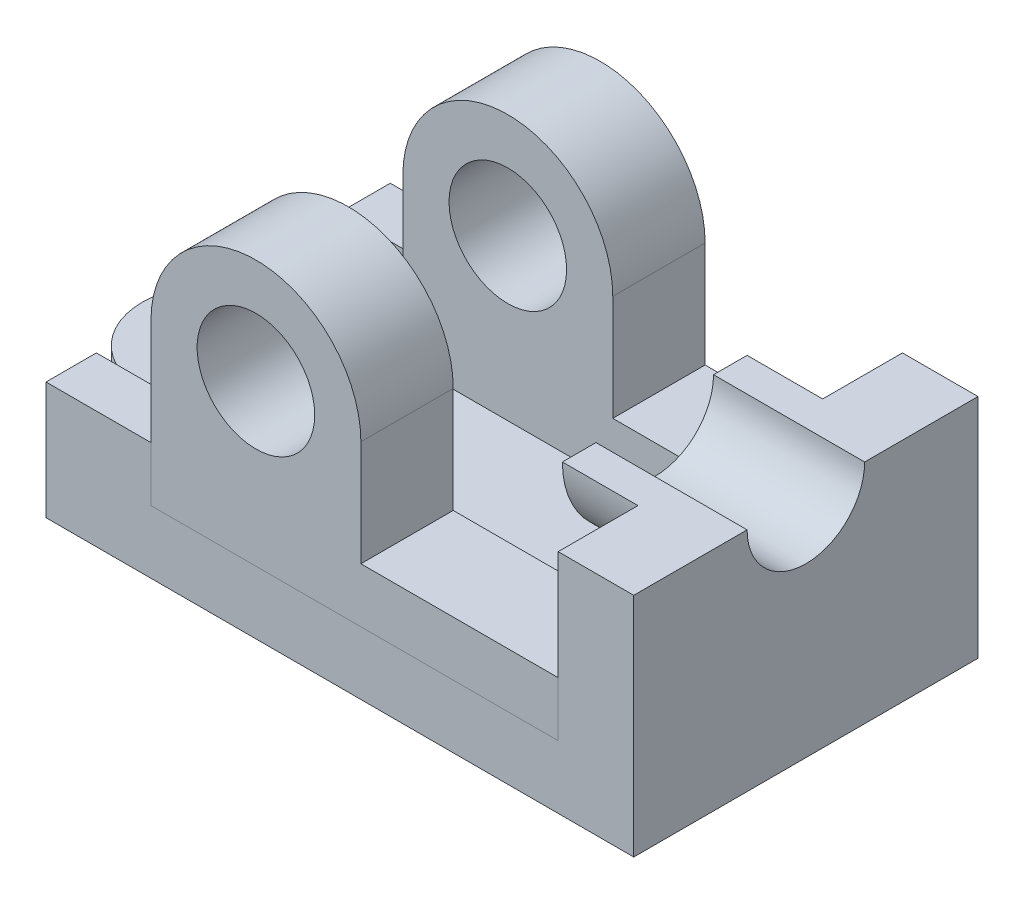
ISO-10303-21;
HEADER;
FILE_DESCRIPTION(('STEP AP214'),'2;1');
FILE_NAME('part.step','',(''),(''),'','','');
FILE_SCHEMA(('AUTOMOTIVE_DESIGN { 1 0 10303 214 1 1 1 1 }'));
ENDSEC;
DATA;
#1=APPLICATION_CONTEXT('core data for automotive mechanical design processes');
#2=APPLICATION_PROTOCOL_DEFINITION('international standard','automotive_design',2000,#1);
#3=PRODUCT_CONTEXT('',#1,'mechanical');
#4=PRODUCT('Part','Part','',(#3));
#5=PRODUCT_RELATED_PRODUCT_CATEGORY('part','',(#4));
#6=PRODUCT_DEFINITION_FORMATION('','',#4);
#7=PRODUCT_DEFINITION_CONTEXT('part definition',#1,'design');
#8=PRODUCT_DEFINITION('design','',#6,#7);
#9=PRODUCT_DEFINITION_SHAPE('','',#8);
#10=(LENGTH_UNIT() NAMED_UNIT(*) SI_UNIT(.MILLI.,.METRE.));
#11=(NAMED_UNIT(*) PLANE_ANGLE_UNIT() SI_UNIT($,.RADIAN.));
#12=(NAMED_UNIT(*) SI_UNIT($,.STERADIAN.) SOLID_ANGLE_UNIT());
#13=UNCERTAINTY_MEASURE_WITH_UNIT(LENGTH_MEASURE(1.E-05),#10,'distance_accuracy_value','');
#14=(GEOMETRIC_REPRESENTATION_CONTEXT(3) GLOBAL_UNCERTAINTY_ASSIGNED_CONTEXT((#13)) GLOBAL_UNIT_ASSIGNED_CONTEXT((#10,
#11,#12)) REPRESENTATION_CONTEXT('',''));
#15=CARTESIAN_POINT('',(0.,0.,0.));
#16=DIRECTION('',(0.,0.,1.));
#17=DIRECTION('',(1.,0.,0.));
#18=AXIS2_PLACEMENT_3D('',#15,#16,#17);
#19=CARTESIAN_POINT('',(-20.,45.6684675281199,19.));
#20=DIRECTION('',(0.,0.,1.));
#21=DIRECTION('',(1.,0.,0.));
#22=AXIS2_PLACEMENT_3D('',#19,#20,#21);
#23=CYLINDRICAL_SURFACE('',#22,25.);
#24=CARTESIAN_POINT('',(-20.,45.6684675281199,41.));
#25=DIRECTION('',(0.,0.,1.));
#26=DIRECTION('',(1.,0.,0.));
#27=AXIS2_PLACEMENT_3D('',#24,#25,#26);
#28=CIRCLE('',#27,25.);
#29=CARTESIAN_POINT('',(5.,45.6684675281199,41.));
#30=VERTEX_POINT('',#29);
#31=CARTESIAN_POINT('',(-45.,45.6684675281199,41.));
#32=VERTEX_POINT('',#31);
#33=EDGE_CURVE('E137',#30,#32,#28,.T.);
#34=ORIENTED_EDGE('',*,*,#33,.F.);
#35=DIRECTION('',(0.,0.,1.));
#36=VECTOR('',#35,1.);
#37=CARTESIAN_POINT('',(5.,45.6684675281199,19.));
#38=LINE('',#37,#36);
#39=CARTESIAN_POINT('',(5.,45.6684675281199,19.));
#40=VERTEX_POINT('',#39);
#41=EDGE_CURVE('E12',#40,#30,#38,.T.);
#42=ORIENTED_EDGE('',*,*,#41,.F.);
#43=CARTESIAN_POINT('',(-20.,45.6684675281199,19.));
#44=DIRECTION('',(0.,0.,1.));
#45=DIRECTION('',(1.,0.,0.));
#46=AXIS2_PLACEMENT_3D('',#43,#44,#45);
#47=CIRCLE('',#46,25.);
#48=CARTESIAN_POINT('',(-45.,45.6684675281199,19.));
#49=VERTEX_POINT('',#48);
#50=EDGE_CURVE('E155',#40,#49,#47,.T.);
#51=ORIENTED_EDGE('',*,*,#50,.T.);
#52=DIRECTION('',(0.,0.,1.));
#53=VECTOR('',#52,1.);
#54=CARTESIAN_POINT('',(-45.,45.6684675281199,19.));
#55=LINE('',#54,#53);
#56=EDGE_CURVE('E103',#49,#32,#55,.T.);
#57=ORIENTED_EDGE('',*,*,#56,.T.);
#58=EDGE_LOOP('',(#34,#42,#51,#57));
#59=FACE_BOUND('',#58,.T.);
#60=ADVANCED_FACE('F51',(#59),#23,.T.);
#61=CARTESIAN_POINT('',(5.,45.6684675281199,19.));
#62=DIRECTION('',(1.,0.,0.));
#63=DIRECTION('',(0.,1.,0.));
#64=AXIS2_PLACEMENT_3D('',#61,#62,#63);
#65=PLANE('',#64);
#66=DIRECTION('',(0.,1.,0.));
#67=VECTOR('',#66,1.);
#68=CARTESIAN_POINT('',(5.,45.6684675281199,41.));
#69=LINE('',#68,#67);
#70=CARTESIAN_POINT('',(5.,20.5,41.));
#71=VERTEX_POINT('',#70);
#72=EDGE_CURVE('E148',#71,#30,#69,.T.);
#73=ORIENTED_EDGE('',*,*,#72,.F.);
#74=DIRECTION('',(0.,0.,1.));
#75=VECTOR('',#74,1.);
#76=CARTESIAN_POINT('',(5.,20.5,19.));
#77=LINE('',#76,#75);
#78=CARTESIAN_POINT('',(5.,20.5,19.));
#79=VERTEX_POINT('',#78);
#80=EDGE_CURVE('E58',#79,#71,#77,.T.);
#81=ORIENTED_EDGE('',*,*,#80,.F.);
#82=DIRECTION('',(0.,1.,0.));
#83=VECTOR('',#82,1.);
#84=CARTESIAN_POINT('',(5.,45.6684675281199,19.));
#85=LINE('',#84,#83);
#86=EDGE_CURVE('E130',#79,#40,#85,.T.);
#87=ORIENTED_EDGE('',*,*,#86,.T.);
#88=ORIENTED_EDGE('',*,*,#41,.T.);
#89=EDGE_LOOP('',(#73,#81,#87,#88));
#90=FACE_BOUND('',#89,.T.);
#91=ADVANCED_FACE('F163',(#90),#65,.T.);
#92=CARTESIAN_POINT('',(5.,20.5,19.));
#93=DIRECTION('',(0.,1.,0.));
#94=DIRECTION('',(0.,0.,1.));
#95=AXIS2_PLACEMENT_3D('',#92,#93,#94);
#96=PLANE('',#95);
#97=DIRECTION('',(-1.,0.,0.));
#98=VECTOR('',#97,1.);
#99=CARTESIAN_POINT('',(5.,20.5,41.));
#100=LINE('',#99,#98);
#101=CARTESIAN_POINT('',(52.,20.5,41.));
#102=VERTEX_POINT('',#101);
#103=EDGE_CURVE('E112',#102,#71,#100,.T.);
#104=ORIENTED_EDGE('',*,*,#103,.F.);
#105=DIRECTION('',(0.,0.,1.));
#106=VECTOR('',#105,1.);
#107=CARTESIAN_POINT('',(52.,20.5,19.));
#108=LINE('',#107,#106);
#109=CARTESIAN_POINT('',(52.,20.5,19.));
#110=VERTEX_POINT('',#109);
#111=EDGE_CURVE('E107',#110,#102,#108,.T.);
#112=ORIENTED_EDGE('',*,*,#111,.F.);
#113=DIRECTION('',(-1.,0.,0.));
#114=VECTOR('',#113,1.);
#115=CARTESIAN_POINT('',(5.,20.5,19.));
#116=LINE('',#115,#114);
#117=EDGE_CURVE('E115',#110,#79,#116,.T.);
#118=ORIENTED_EDGE('',*,*,#117,.T.);
#119=ORIENTED_EDGE('',*,*,#80,.T.);
#120=EDGE_LOOP('',(#104,#112,#118,#119));
#121=FACE_BOUND('',#120,.T.);
#122=ADVANCED_FACE('F111',(#121),#96,.T.);
#123=CARTESIAN_POINT('',(52.,20.5,19.));
#124=DIRECTION('',(1.,0.,0.));
#125=DIRECTION('',(0.,0.,-1.));
#126=AXIS2_PLACEMENT_3D('',#123,#124,#125);
#127=PLANE('',#126);
#128=DIRECTION('',(0.,1.,0.));
#129=VECTOR('',#128,1.);
#130=CARTESIAN_POINT('',(52.,20.5,41.));
#131=LINE('',#130,#129);
#132=CARTESIAN_POINT('',(52.,7.5,41.));
#133=VERTEX_POINT('',#132);
#134=EDGE_CURVE('E150',#133,#102,#131,.T.);
#135=ORIENTED_EDGE('',*,*,#134,.F.);
#136=DIRECTION('',(0.,0.,1.));
#137=VECTOR('',#136,1.);
#138=CARTESIAN_POINT('',(52.,7.5,19.));
#139=LINE('',#138,#137);
#140=CARTESIAN_POINT('',(52.,7.5,19.));
#141=VERTEX_POINT('',#140);
#142=EDGE_CURVE('E118',#141,#133,#139,.T.);
#143=ORIENTED_EDGE('',*,*,#142,.F.);
#144=DIRECTION('',(0.,1.,0.));
#145=VECTOR('',#144,1.);
#146=CARTESIAN_POINT('',(52.,20.5,19.));
#147=LINE('',#146,#145);
#148=EDGE_CURVE('E123',#141,#110,#147,.T.);
#149=ORIENTED_EDGE('',*,*,#148,.T.);
#150=ORIENTED_EDGE('',*,*,#111,.T.);
#151=EDGE_LOOP('',(#135,#143,#149,#150));
#152=FACE_BOUND('',#151,.T.);
#153=ADVANCED_FACE('F126',(#152),#127,.T.);
#154=CARTESIAN_POINT('',(52.,7.5,19.));
#155=DIRECTION('',(0.,-1.,0.));
#156=DIRECTION('',(0.,0.,-1.));
#157=AXIS2_PLACEMENT_3D('',#154,#155,#156);
#158=PLANE('',#157);
#159=DIRECTION('',(1.,0.,0.));
#160=VECTOR('',#159,1.);
#161=CARTESIAN_POINT('',(52.,7.5,41.));
#162=LINE('',#161,#160);
#163=CARTESIAN_POINT('',(-45.,7.5,41.));
#164=VERTEX_POINT('',#163);
#165=EDGE_CURVE('E144',#164,#133,#162,.T.);
#166=ORIENTED_EDGE('',*,*,#165,.F.);
#167=DIRECTION('',(0.,0.,1.));
#168=VECTOR('',#167,1.);
#169=CARTESIAN_POINT('',(-45.,7.5,19.));
#170=LINE('',#169,#168);
#171=CARTESIAN_POINT('',(-45.,7.5,19.));
#172=VERTEX_POINT('',#171);
#173=EDGE_CURVE('E156',#172,#164,#170,.T.);
#174=ORIENTED_EDGE('',*,*,#173,.F.);
#175=DIRECTION('',(1.,0.,0.));
#176=VECTOR('',#175,1.);
#177=CARTESIAN_POINT('',(52.,7.5,19.));
#178=LINE('',#177,#176);
#179=EDGE_CURVE('E128',#172,#141,#178,.T.);
#180=ORIENTED_EDGE('',*,*,#179,.T.);
#181=ORIENTED_EDGE('',*,*,#142,.T.);
#182=EDGE_LOOP('',(#166,#174,#180,#181));
#183=FACE_BOUND('',#182,.T.);
#184=ADVANCED_FACE('F172',(#183),#158,.T.);
#185=CARTESIAN_POINT('',(-45.,45.6684675281199,19.));
#186=DIRECTION('',(-1.,0.,0.));
#187=DIRECTION('',(0.,0.,1.));
#188=AXIS2_PLACEMENT_3D('',#185,#186,#187);
#189=PLANE('',#188);
#190=DIRECTION('',(0.,-1.,0.));
#191=VECTOR('',#190,1.);
#192=CARTESIAN_POINT('',(-45.,45.6684675281199,41.));
#193=LINE('',#192,#191);
#194=EDGE_CURVE('E140',#32,#164,#193,.T.);
#195=ORIENTED_EDGE('',*,*,#194,.F.);
#196=ORIENTED_EDGE('',*,*,#56,.F.);
#197=DIRECTION('',(0.,-1.,0.));
#198=VECTOR('',#197,1.);
#199=CARTESIAN_POINT('',(-45.,45.6684675281199,19.));
#200=LINE('',#199,#198);
#201=EDGE_CURVE('E135',#49,#172,#200,.T.);
#202=ORIENTED_EDGE('',*,*,#201,.T.);
#203=ORIENTED_EDGE('',*,*,#173,.T.);
#204=EDGE_LOOP('',(#195,#196,#202,#203));
#205=FACE_BOUND('',#204,.T.);
#206=ADVANCED_FACE('F157',(#205),#189,.T.);
#207=CARTESIAN_POINT('',(-20.,45.6684675281199,19.));
#208=DIRECTION('',(0.,0.,1.));
#209=DIRECTION('',(1.,0.,0.));
#210=AXIS2_PLACEMENT_3D('',#207,#208,#209);
#211=PLANE('',#210);
#212=CARTESIAN_POINT('',(-20.,45.6684675281199,19.));
#213=DIRECTION('',(0.,0.,1.));
#214=DIRECTION('',(1.,0.,0.));
#215=AXIS2_PLACEMENT_3D('',#212,#213,#214);
#216=CIRCLE('',#215,14.);
#217=CARTESIAN_POINT('',(-6.,45.6684675281199,19.));
#218=VERTEX_POINT('',#217);
#219=EDGE_CURVE('E142',#218,#218,#216,.T.);
#220=ORIENTED_EDGE('',*,*,#219,.T.);
#221=EDGE_LOOP('',(#220));
#222=FACE_BOUND('',#221,.T.);
#223=ORIENTED_EDGE('',*,*,#50,.F.);
#224=ORIENTED_EDGE('',*,*,#86,.F.);
#225=ORIENTED_EDGE('',*,*,#117,.F.);
#226=ORIENTED_EDGE('',*,*,#148,.F.);
#227=ORIENTED_EDGE('',*,*,#179,.F.);
#228=ORIENTED_EDGE('',*,*,#201,.F.);
#229=EDGE_LOOP('',(#223,#224,#225,#226,#227,#228));
#230=FACE_BOUND('',#229,.T.);
#231=ADVANCED_FACE('F124',(#222,#230),#211,.F.);
#232=CARTESIAN_POINT('',(-20.,45.6684675281199,41.));
#233=DIRECTION('',(0.,0.,1.));
#234=DIRECTION('',(1.,0.,0.));
#235=AXIS2_PLACEMENT_3D('',#232,#233,#234);
#236=PLANE('',#235);
#237=CARTESIAN_POINT('',(-20.,45.6684675281199,41.));
#238=DIRECTION('',(0.,0.,1.));
#239=DIRECTION('',(1.,0.,0.));
#240=AXIS2_PLACEMENT_3D('',#237,#238,#239);
#241=CIRCLE('',#240,14.);
#242=CARTESIAN_POINT('',(-6.,45.6684675281199,41.));
#243=VERTEX_POINT('',#242);
#244=EDGE_CURVE('E53',#243,#243,#241,.T.);
#245=ORIENTED_EDGE('',*,*,#244,.F.);
#246=EDGE_LOOP('',(#245));
#247=FACE_BOUND('',#246,.T.);
#248=ORIENTED_EDGE('',*,*,#33,.T.);
#249=ORIENTED_EDGE('',*,*,#194,.T.);
#250=ORIENTED_EDGE('',*,*,#165,.T.);
#251=ORIENTED_EDGE('',*,*,#134,.T.);
#252=ORIENTED_EDGE('',*,*,#103,.T.);
#253=ORIENTED_EDGE('',*,*,#72,.T.);
#254=EDGE_LOOP('',(#248,#249,#250,#251,#252,#253));
#255=FACE_BOUND('',#254,.T.);
#256=ADVANCED_FACE('F160',(#247,#255),#236,.T.);
#257=CARTESIAN_POINT('',(-20.,45.6684675281199,-41.));
#258=DIRECTION('',(0.,0.,1.));
#259=DIRECTION('',(1.,0.,0.));
#260=AXIS2_PLACEMENT_3D('',#257,#258,#259);
#261=CYLINDRICAL_SURFACE('',#260,14.);
#262=ORIENTED_EDGE('',*,*,#244,.T.);
#263=EDGE_LOOP('',(#262));
#264=FACE_BOUND('',#263,.T.);
#265=ORIENTED_EDGE('',*,*,#219,.F.);
#266=EDGE_LOOP('',(#265));
#267=FACE_BOUND('',#266,.T.);
#268=ADVANCED_FACE('F184',(#264,#267),#261,.F.);
#269=CLOSED_SHELL('',(#60,#91,#122,#153,#184,#206,#231,#256,#268));
#270=MANIFOLD_SOLID_BREP('B2',#269);
#271=CARTESIAN_POINT('',(-70.,7.5,-41.));
#272=DIRECTION('',(1.,0.,0.));
#273=DIRECTION('',(0.,0.,-1.));
#274=AXIS2_PLACEMENT_3D('',#271,#272,#273);
#275=PLANE('',#274);
#276=DIRECTION('',(0.,0.,1.));
#277=VECTOR('',#276,1.);
#278=CARTESIAN_POINT('',(-70.,-7.5,-41.));
#279=LINE('',#278,#277);
#280=CARTESIAN_POINT('',(-70.,-7.5,-41.));
#281=VERTEX_POINT('',#280);
#282=CARTESIAN_POINT('',(-70.,-7.5,-18.));
#283=VERTEX_POINT('',#282);
#284=EDGE_CURVE('E418',#281,#283,#279,.T.);
#285=ORIENTED_EDGE('',*,*,#284,.T.);
#286=DIRECTION('',(0.,1.,0.));
#287=VECTOR('',#286,1.);
#288=CARTESIAN_POINT('',(-70.,-7.5,-18.));
#289=LINE('',#288,#287);
#290=CARTESIAN_POINT('',(-70.,7.5,-18.));
#291=VERTEX_POINT('',#290);
#292=EDGE_CURVE('E405',#283,#291,#289,.T.);
#293=ORIENTED_EDGE('',*,*,#292,.T.);
#294=DIRECTION('',(0.,0.,1.));
#295=VECTOR('',#294,1.);
#296=CARTESIAN_POINT('',(-70.,7.5,-41.));
#297=LINE('',#296,#295);
#298=CARTESIAN_POINT('',(-70.,7.5,-29.));
#299=VERTEX_POINT('',#298);
#300=EDGE_CURVE('E572',#299,#291,#297,.T.);
#301=ORIENTED_EDGE('',*,*,#300,.F.);
#302=DIRECTION('',(0.,-1.,0.));
#303=VECTOR('',#302,1.);
#304=CARTESIAN_POINT('',(-70.,20.5,-29.));
#305=LINE('',#304,#303);
#306=CARTESIAN_POINT('',(-70.,20.5,-29.));
#307=VERTEX_POINT('',#306);
#308=EDGE_CURVE('E465',#307,#299,#305,.T.);
#309=ORIENTED_EDGE('',*,*,#308,.F.);
#310=DIRECTION('',(0.,0.,-1.));
#311=VECTOR('',#310,1.);
#312=CARTESIAN_POINT('',(-70.,20.5,0.));
#313=LINE('',#312,#311);
#314=CARTESIAN_POINT('',(-70.,20.5,-41.));
#315=VERTEX_POINT('',#314);
#316=EDGE_CURVE('E460',#307,#315,#313,.T.);
#317=ORIENTED_EDGE('',*,*,#316,.T.);
#318=DIRECTION('',(0.,-1.,0.));
#319=VECTOR('',#318,1.);
#320=CARTESIAN_POINT('',(-70.,7.5,-41.));
#321=LINE('',#320,#319);
#322=EDGE_CURVE('E433',#315,#281,#321,.T.);
#323=ORIENTED_EDGE('',*,*,#322,.T.);
#324=EDGE_LOOP('',(#285,#293,#301,#309,#317,#323));
#325=FACE_BOUND('',#324,.T.);
#326=ADVANCED_FACE('F247',(#325),#275,.F.);
#327=CARTESIAN_POINT('',(0.,7.5,0.));
#328=DIRECTION('',(0.,1.,0.));
#329=DIRECTION('',(0.,0.,1.));
#330=AXIS2_PLACEMENT_3D('',#327,#328,#329);
#331=PLANE('',#330);
#332=CARTESIAN_POINT('',(-70.,7.5,0.));
#333=DIRECTION('',(0.,1.,0.));
#334=DIRECTION('',(0.,0.,1.));
#335=AXIS2_PLACEMENT_3D('',#332,#333,#334);
#336=CIRCLE('',#335,11.);
#337=CARTESIAN_POINT('',(-70.,7.5,11.));
#338=VERTEX_POINT('',#337);
#339=EDGE_CURVE('E656',#338,#338,#336,.T.);
#340=ORIENTED_EDGE('',*,*,#339,.F.);
#341=EDGE_LOOP('',(#340));
#342=FACE_BOUND('',#341,.T.);
#343=ORIENTED_EDGE('',*,*,#300,.T.);
#344=CARTESIAN_POINT('',(-70.,7.5,0.));
#345=DIRECTION('',(0.,1.,0.));
#346=DIRECTION('',(0.,0.,1.));
#347=AXIS2_PLACEMENT_3D('',#344,#345,#346);
#348=CIRCLE('',#347,18.);
#349=CARTESIAN_POINT('',(-70.,7.5,18.));
#350=VERTEX_POINT('',#349);
#351=EDGE_CURVE('E262',#291,#350,#348,.T.);
#352=ORIENTED_EDGE('',*,*,#351,.T.);
#353=CARTESIAN_POINT('',(-70.,7.5,29.));
#354=VERTEX_POINT('',#353);
#355=EDGE_CURVE('E411',#350,#354,#297,.T.);
#356=ORIENTED_EDGE('',*,*,#355,.T.);
#357=DIRECTION('',(1.,0.,0.));
#358=VECTOR('',#357,1.);
#359=CARTESIAN_POINT('',(0.,7.5,29.));
#360=LINE('',#359,#358);
#361=CARTESIAN_POINT('',(-36.2,7.5,29.));
#362=VERTEX_POINT('',#361);
#363=EDGE_CURVE('E512',#354,#362,#360,.T.);
#364=ORIENTED_EDGE('',*,*,#363,.T.);
#365=DIRECTION('',(0.,0.,-1.));
#366=VECTOR('',#365,1.);
#367=CARTESIAN_POINT('',(-36.2,7.5,0.));
#368=LINE('',#367,#366);
#369=CARTESIAN_POINT('',(-36.2,7.5,41.));
#370=VERTEX_POINT('',#369);
#371=EDGE_CURVE('E506',#370,#362,#368,.T.);
#372=ORIENTED_EDGE('',*,*,#371,.F.);
#373=DIRECTION('',(1.,0.,0.));
#374=VECTOR('',#373,1.);
#375=CARTESIAN_POINT('',(-70.,7.5,41.));
#376=LINE('',#375,#374);
#377=CARTESIAN_POINT('',(52.,7.5,41.));
#378=VERTEX_POINT('',#377);
#379=EDGE_CURVE('E431',#370,#378,#376,.T.);
#380=ORIENTED_EDGE('',*,*,#379,.T.);
#381=DIRECTION('',(0.,0.,1.));
#382=VECTOR('',#381,1.);
#383=CARTESIAN_POINT('',(52.,7.5,-41.));
#384=LINE('',#383,#382);
#385=CARTESIAN_POINT('',(52.,7.5,-19.));
#386=VERTEX_POINT('',#385);
#387=EDGE_CURVE('E551',#386,#378,#384,.T.);
#388=ORIENTED_EDGE('',*,*,#387,.F.);
#389=DIRECTION('',(1.,0.,0.));
#390=VECTOR('',#389,1.);
#391=CARTESIAN_POINT('',(52.,7.5,-19.));
#392=LINE('',#391,#390);
#393=CARTESIAN_POINT('',(-45.,7.5,-19.));
#394=VERTEX_POINT('',#393);
#395=EDGE_CURVE('E497',#394,#386,#392,.T.);
#396=ORIENTED_EDGE('',*,*,#395,.F.);
#397=DIRECTION('',(0.,0.,-1.));
#398=VECTOR('',#397,1.);
#399=CARTESIAN_POINT('',(-45.,7.5,-19.));
#400=LINE('',#399,#398);
#401=CARTESIAN_POINT('',(-45.,7.5,-29.));
#402=VERTEX_POINT('',#401);
#403=EDGE_CURVE('E500',#394,#402,#400,.T.);
#404=ORIENTED_EDGE('',*,*,#403,.T.);
#405=DIRECTION('',(1.,0.,0.));
#406=VECTOR('',#405,1.);
#407=CARTESIAN_POINT('',(0.,7.5,-29.));
#408=LINE('',#407,#406);
#409=EDGE_CURVE('E270',#299,#402,#408,.T.);
#410=ORIENTED_EDGE('',*,*,#409,.F.);
#411=EDGE_LOOP('',(#343,#352,#356,#364,#372,#380,#388,#396,#404,#410));
#412=FACE_BOUND('',#411,.T.);
#413=ADVANCED_FACE('F611',(#342,#412),#331,.T.);
#414=CARTESIAN_POINT('',(-45.,45.6684675281199,-19.));
#415=DIRECTION('',(-1.,0.,0.));
#416=DIRECTION('',(0.,0.,-1.));
#417=AXIS2_PLACEMENT_3D('',#414,#415,#416);
#418=PLANE('',#417);
#419=DIRECTION('',(0.,0.,-1.));
#420=VECTOR('',#419,1.);
#421=CARTESIAN_POINT('',(-45.,20.5,-19.));
#422=LINE('',#421,#420);
#423=CARTESIAN_POINT('',(-45.,20.5,-29.));
#424=VERTEX_POINT('',#423);
#425=CARTESIAN_POINT('',(-45.,20.5,-41.));
#426=VERTEX_POINT('',#425);
#427=EDGE_CURVE('E260',#424,#426,#422,.T.);
#428=ORIENTED_EDGE('',*,*,#427,.F.);
#429=DIRECTION('',(0.,-1.,0.));
#430=VECTOR('',#429,1.);
#431=CARTESIAN_POINT('',(-45.,45.6684675281199,-29.));
#432=LINE('',#431,#430);
#433=EDGE_CURVE('E47',#424,#402,#432,.T.);
#434=ORIENTED_EDGE('',*,*,#433,.T.);
#435=ORIENTED_EDGE('',*,*,#403,.F.);
#436=DIRECTION('',(0.,-1.,0.));
#437=VECTOR('',#436,1.);
#438=CARTESIAN_POINT('',(-45.,45.6684675281199,-19.));
#439=LINE('',#438,#437);
#440=CARTESIAN_POINT('',(-45.,45.6684675281199,-19.));
#441=VERTEX_POINT('',#440);
#442=EDGE_CURVE('E503',#441,#394,#439,.T.);
#443=ORIENTED_EDGE('',*,*,#442,.F.);
#444=DIRECTION('',(0.,0.,-1.));
#445=VECTOR('',#444,1.);
#446=CARTESIAN_POINT('',(-45.,45.6684675281199,-19.));
#447=LINE('',#446,#445);
#448=CARTESIAN_POINT('',(-45.,45.6684675281199,-41.));
#449=VERTEX_POINT('',#448);
#450=EDGE_CURVE('E476',#441,#449,#447,.T.);
#451=ORIENTED_EDGE('',*,*,#450,.T.);
#452=DIRECTION('',(0.,-1.,0.));
#453=VECTOR('',#452,1.);
#454=CARTESIAN_POINT('',(-45.,45.6684675281199,-41.));
#455=LINE('',#454,#453);
#456=EDGE_CURVE('E453',#449,#426,#455,.T.);
#457=ORIENTED_EDGE('',*,*,#456,.T.);
#458=EDGE_LOOP('',(#428,#434,#435,#443,#451,#457));
#459=FACE_BOUND('',#458,.T.);
#460=ADVANCED_FACE('F634',(#459),#418,.T.);
#461=CARTESIAN_POINT('',(0.,46.5,0.));
#462=DIRECTION('',(0.,-1.,0.));
#463=DIRECTION('',(0.,0.,-1.));
#464=AXIS2_PLACEMENT_3D('',#461,#462,#463);
#465=PLANE('',#464);
#466=DIRECTION('',(1.,0.,0.));
#467=VECTOR('',#466,1.);
#468=CARTESIAN_POINT('',(34.,46.5,-14.));
#469=LINE('',#468,#467);
#470=CARTESIAN_POINT('',(34.,46.5,-14.));
#471=VERTEX_POINT('',#470);
#472=CARTESIAN_POINT('',(70.,46.5,-14.));
#473=VERTEX_POINT('',#472);
#474=EDGE_CURVE('E541',#471,#473,#469,.T.);
#475=ORIENTED_EDGE('',*,*,#474,.T.);
#476=DIRECTION('',(0.,0.,-1.));
#477=VECTOR('',#476,1.);
#478=CARTESIAN_POINT('',(70.,46.5,-41.));
#479=LINE('',#478,#477);
#480=CARTESIAN_POINT('',(70.,46.5,-41.));
#481=VERTEX_POINT('',#480);
#482=EDGE_CURVE('E556',#473,#481,#479,.T.);
#483=ORIENTED_EDGE('',*,*,#482,.T.);
#484=DIRECTION('',(-1.,0.,0.));
#485=VECTOR('',#484,1.);
#486=CARTESIAN_POINT('',(70.,46.5,-41.));
#487=LINE('',#486,#485);
#488=CARTESIAN_POINT('',(52.,46.5,-41.));
#489=VERTEX_POINT('',#488);
#490=EDGE_CURVE('E560',#481,#489,#487,.T.);
#491=ORIENTED_EDGE('',*,*,#490,.T.);
#492=DIRECTION('',(0.,0.,1.));
#493=VECTOR('',#492,1.);
#494=CARTESIAN_POINT('',(52.,46.5,-41.));
#495=LINE('',#494,#493);
#496=CARTESIAN_POINT('',(52.,46.5,-22.));
#497=VERTEX_POINT('',#496);
#498=EDGE_CURVE('E561',#489,#497,#495,.T.);
#499=ORIENTED_EDGE('',*,*,#498,.T.);
#500=DIRECTION('',(1.,0.,0.));
#501=VECTOR('',#500,1.);
#502=CARTESIAN_POINT('',(34.,46.5,-22.));
#503=LINE('',#502,#501);
#504=CARTESIAN_POINT('',(34.,46.5,-22.));
#505=VERTEX_POINT('',#504);
#506=EDGE_CURVE('E553',#505,#497,#503,.T.);
#507=ORIENTED_EDGE('',*,*,#506,.F.);
#508=DIRECTION('',(0.,0.,-1.));
#509=VECTOR('',#508,1.);
#510=CARTESIAN_POINT('',(34.,46.5,0.));
#511=LINE('',#510,#509);
#512=EDGE_CURVE('E534',#471,#505,#511,.T.);
#513=ORIENTED_EDGE('',*,*,#512,.F.);
#514=EDGE_LOOP('',(#475,#483,#491,#499,#507,#513));
#515=FACE_BOUND('',#514,.T.);
#516=ADVANCED_FACE('F588',(#515),#465,.F.);
#517=CARTESIAN_POINT('',(70.,7.5,-41.));
#518=DIRECTION('',(-1.,0.,0.));
#519=DIRECTION('',(0.,0.,1.));
#520=AXIS2_PLACEMENT_3D('',#517,#518,#519);
#521=PLANE('',#520);
#522=ORIENTED_EDGE('',*,*,#482,.F.);
#523=CARTESIAN_POINT('',(70.,46.5,0.));
#524=DIRECTION('',(1.,0.,0.));
#525=DIRECTION('',(0.,0.,-1.));
#526=AXIS2_PLACEMENT_3D('',#523,#524,#525);
#527=CIRCLE('',#526,14.);
#528=CARTESIAN_POINT('',(70.,46.5,14.));
#529=VERTEX_POINT('',#528);
#530=EDGE_CURVE('E530',#529,#473,#527,.T.);
#531=ORIENTED_EDGE('',*,*,#530,.F.);
#532=CARTESIAN_POINT('',(70.,46.5,41.));
#533=VERTEX_POINT('',#532);
#534=EDGE_CURVE('E555',#533,#529,#479,.T.);
#535=ORIENTED_EDGE('',*,*,#534,.F.);
#536=DIRECTION('',(0.,-1.,0.));
#537=VECTOR('',#536,1.);
#538=CARTESIAN_POINT('',(70.,7.5,41.));
#539=LINE('',#538,#537);
#540=CARTESIAN_POINT('',(70.,-7.5,41.));
#541=VERTEX_POINT('',#540);
#542=EDGE_CURVE('E430',#533,#541,#539,.T.);
#543=ORIENTED_EDGE('',*,*,#542,.T.);
#544=DIRECTION('',(0.,0.,-1.));
#545=VECTOR('',#544,1.);
#546=CARTESIAN_POINT('',(70.,-7.5,-41.));
#547=LINE('',#546,#545);
#548=CARTESIAN_POINT('',(70.,-7.5,-41.));
#549=VERTEX_POINT('',#548);
#550=EDGE_CURVE('E422',#541,#549,#547,.T.);
#551=ORIENTED_EDGE('',*,*,#550,.T.);
#552=DIRECTION('',(0.,-1.,0.));
#553=VECTOR('',#552,1.);
#554=CARTESIAN_POINT('',(70.,7.5,-41.));
#555=LINE('',#554,#553);
#556=EDGE_CURVE('E436',#481,#549,#555,.T.);
#557=ORIENTED_EDGE('',*,*,#556,.F.);
#558=EDGE_LOOP('',(#522,#531,#535,#543,#551,#557));
#559=FACE_BOUND('',#558,.T.);
#560=ADVANCED_FACE('F249',(#559),#521,.F.);
#561=CARTESIAN_POINT('',(-70.,7.5,-41.));
#562=DIRECTION('',(0.,0.,1.));
#563=DIRECTION('',(1.,0.,0.));
#564=AXIS2_PLACEMENT_3D('',#561,#562,#563);
#565=PLANE('',#564);
#566=CARTESIAN_POINT('',(-20.,45.6684675281199,-41.));
#567=DIRECTION('',(0.,0.,1.));
#568=DIRECTION('',(1.,0.,0.));
#569=AXIS2_PLACEMENT_3D('',#566,#567,#568);
#570=CIRCLE('',#569,14.);
#571=CARTESIAN_POINT('',(-6.,45.6684675281199,-41.));
#572=VERTEX_POINT('',#571);
#573=EDGE_CURVE('E462',#572,#572,#570,.T.);
#574=ORIENTED_EDGE('',*,*,#573,.T.);
#575=EDGE_LOOP('',(#574));
#576=FACE_BOUND('',#575,.T.);
#577=DIRECTION('',(1.,0.,0.));
#578=VECTOR('',#577,1.);
#579=CARTESIAN_POINT('',(0.,20.5,-41.));
#580=LINE('',#579,#578);
#581=EDGE_CURVE('E447',#315,#426,#580,.T.);
#582=ORIENTED_EDGE('',*,*,#581,.T.);
#583=ORIENTED_EDGE('',*,*,#456,.F.);
#584=CARTESIAN_POINT('',(-20.,45.6684675281199,-41.));
#585=DIRECTION('',(0.,0.,1.));
#586=DIRECTION('',(1.,0.,0.));
#587=AXIS2_PLACEMENT_3D('',#584,#585,#586);
#588=CIRCLE('',#587,25.);
#589=CARTESIAN_POINT('',(5.,45.6684675281199,-41.));
#590=VERTEX_POINT('',#589);
#591=EDGE_CURVE('E469',#590,#449,#588,.T.);
#592=ORIENTED_EDGE('',*,*,#591,.F.);
#593=DIRECTION('',(0.,1.,0.));
#594=VECTOR('',#593,1.);
#595=CARTESIAN_POINT('',(5.,45.6684675281199,-41.));
#596=LINE('',#595,#594);
#597=CARTESIAN_POINT('',(5.,20.5,-41.));
#598=VERTEX_POINT('',#597);
#599=EDGE_CURVE('E479',#598,#590,#596,.T.);
#600=ORIENTED_EDGE('',*,*,#599,.F.);
#601=DIRECTION('',(-1.,0.,0.));
#602=VECTOR('',#601,1.);
#603=CARTESIAN_POINT('',(5.,20.5,-41.));
#604=LINE('',#603,#602);
#605=CARTESIAN_POINT('',(52.,20.5,-41.));
#606=VERTEX_POINT('',#605);
#607=EDGE_CURVE('E487',#606,#598,#604,.T.);
#608=ORIENTED_EDGE('',*,*,#607,.F.);
#609=DIRECTION('',(0.,-1.,0.));
#610=VECTOR('',#609,1.);
#611=CARTESIAN_POINT('',(52.,46.5,-41.));
#612=LINE('',#611,#610);
#613=EDGE_CURVE('E571',#489,#606,#612,.T.);
#614=ORIENTED_EDGE('',*,*,#613,.F.);
#615=ORIENTED_EDGE('',*,*,#490,.F.);
#616=ORIENTED_EDGE('',*,*,#556,.T.);
#617=DIRECTION('',(-1.,0.,0.));
#618=VECTOR('',#617,1.);
#619=CARTESIAN_POINT('',(-70.,-7.5,-41.));
#620=LINE('',#619,#618);
#621=EDGE_CURVE('E420',#549,#281,#620,.T.);
#622=ORIENTED_EDGE('',*,*,#621,.T.);
#623=ORIENTED_EDGE('',*,*,#322,.F.);
#624=EDGE_LOOP('',(#582,#583,#592,#600,#608,#614,#615,#616,#622,#623));
#625=FACE_BOUND('',#624,.T.);
#626=ADVANCED_FACE('F454',(#576,#625),#565,.F.);
#627=ORIENTED_EDGE('',*,*,#355,.F.);
#628=DIRECTION('',(0.,1.,0.));
#629=VECTOR('',#628,1.);
#630=CARTESIAN_POINT('',(-70.,-7.5,18.));
#631=LINE('',#630,#629);
#632=CARTESIAN_POINT('',(-70.,-7.5,18.));
#633=VERTEX_POINT('',#632);
#634=EDGE_CURVE('E398',#350,#633,#631,.F.);
#635=ORIENTED_EDGE('',*,*,#634,.T.);
#636=CARTESIAN_POINT('',(-70.,-7.5,41.));
#637=VERTEX_POINT('',#636);
#638=EDGE_CURVE('E408',#633,#637,#279,.T.);
#639=ORIENTED_EDGE('',*,*,#638,.T.);
#640=DIRECTION('',(0.,-1.,0.));
#641=VECTOR('',#640,1.);
#642=CARTESIAN_POINT('',(-70.,7.5,41.));
#643=LINE('',#642,#641);
#644=CARTESIAN_POINT('',(-70.,20.5,41.));
#645=VERTEX_POINT('',#644);
#646=EDGE_CURVE('E427',#645,#637,#643,.T.);
#647=ORIENTED_EDGE('',*,*,#646,.F.);
#648=DIRECTION('',(0.,0.,1.));
#649=VECTOR('',#648,1.);
#650=CARTESIAN_POINT('',(-70.,20.5,0.));
#651=LINE('',#650,#649);
#652=CARTESIAN_POINT('',(-70.,20.5,29.));
#653=VERTEX_POINT('',#652);
#654=EDGE_CURVE('E517',#653,#645,#651,.T.);
#655=ORIENTED_EDGE('',*,*,#654,.F.);
#656=DIRECTION('',(0.,-1.,0.));
#657=VECTOR('',#656,1.);
#658=CARTESIAN_POINT('',(-70.,20.5,29.));
#659=LINE('',#658,#657);
#660=EDGE_CURVE('E516',#653,#354,#659,.T.);
#661=ORIENTED_EDGE('',*,*,#660,.T.);
#662=EDGE_LOOP('',(#627,#635,#639,#647,#655,#661));
#663=FACE_BOUND('',#662,.T.);
#664=ADVANCED_FACE('F406',(#663),#275,.F.);
#665=CARTESIAN_POINT('',(-70.,7.5,41.));
#666=DIRECTION('',(0.,0.,-1.));
#667=DIRECTION('',(-1.,0.,0.));
#668=AXIS2_PLACEMENT_3D('',#665,#666,#667);
#669=PLANE('',#668);
#670=DIRECTION('',(1.,0.,0.));
#671=VECTOR('',#670,1.);
#672=CARTESIAN_POINT('',(-70.,-7.5,41.));
#673=LINE('',#672,#671);
#674=EDGE_CURVE('E419',#637,#541,#673,.T.);
#675=ORIENTED_EDGE('',*,*,#674,.T.);
#676=ORIENTED_EDGE('',*,*,#542,.F.);
#677=DIRECTION('',(1.,0.,0.));
#678=VECTOR('',#677,1.);
#679=CARTESIAN_POINT('',(70.,46.5,41.));
#680=LINE('',#679,#678);
#681=CARTESIAN_POINT('',(52.,46.5,41.));
#682=VERTEX_POINT('',#681);
#683=EDGE_CURVE('E562',#682,#533,#680,.T.);
#684=ORIENTED_EDGE('',*,*,#683,.F.);
#685=DIRECTION('',(0.,-1.,0.));
#686=VECTOR('',#685,1.);
#687=CARTESIAN_POINT('',(52.,46.5,41.));
#688=LINE('',#687,#686);
#689=EDGE_CURVE('E570',#682,#378,#688,.T.);
#690=ORIENTED_EDGE('',*,*,#689,.T.);
#691=ORIENTED_EDGE('',*,*,#379,.F.);
#692=DIRECTION('',(0.,-1.,0.));
#693=VECTOR('',#692,1.);
#694=CARTESIAN_POINT('',(-36.2,20.5,41.));
#695=LINE('',#694,#693);
#696=CARTESIAN_POINT('',(-36.2,20.5,41.));
#697=VERTEX_POINT('',#696);
#698=EDGE_CURVE('E527',#697,#370,#695,.T.);
#699=ORIENTED_EDGE('',*,*,#698,.F.);
#700=DIRECTION('',(1.,0.,0.));
#701=VECTOR('',#700,1.);
#702=CARTESIAN_POINT('',(0.,20.5,41.));
#703=LINE('',#702,#701);
#704=EDGE_CURVE('E510',#645,#697,#703,.T.);
#705=ORIENTED_EDGE('',*,*,#704,.F.);
#706=ORIENTED_EDGE('',*,*,#646,.T.);
#707=EDGE_LOOP('',(#675,#676,#684,#690,#691,#699,#705,#706));
#708=FACE_BOUND('',#707,.T.);
#709=ADVANCED_FACE('F599',(#708),#669,.F.);
#710=CARTESIAN_POINT('',(0.,-7.5,0.));
#711=DIRECTION('',(0.,1.,0.));
#712=DIRECTION('',(0.,0.,1.));
#713=AXIS2_PLACEMENT_3D('',#710,#711,#712);
#714=PLANE('',#713);
#715=CARTESIAN_POINT('',(-70.,-7.5,0.));
#716=DIRECTION('',(0.,1.,0.));
#717=DIRECTION('',(0.,0.,1.));
#718=AXIS2_PLACEMENT_3D('',#715,#716,#717);
#719=CIRCLE('',#718,11.);
#720=CARTESIAN_POINT('',(-70.,-7.5,11.));
#721=VERTEX_POINT('',#720);
#722=EDGE_CURVE('E652',#721,#721,#719,.T.);
#723=ORIENTED_EDGE('',*,*,#722,.T.);
#724=EDGE_LOOP('',(#723));
#725=FACE_BOUND('',#724,.T.);
#726=ORIENTED_EDGE('',*,*,#638,.F.);
#727=CARTESIAN_POINT('',(-70.,-7.5,0.));
#728=DIRECTION('',(0.,1.,0.));
#729=DIRECTION('',(0.,0.,1.));
#730=AXIS2_PLACEMENT_3D('',#727,#728,#729);
#731=CIRCLE('',#730,18.);
#732=EDGE_CURVE('E396',#283,#633,#731,.T.);
#733=ORIENTED_EDGE('',*,*,#732,.F.);
#734=ORIENTED_EDGE('',*,*,#284,.F.);
#735=ORIENTED_EDGE('',*,*,#621,.F.);
#736=ORIENTED_EDGE('',*,*,#550,.F.);
#737=ORIENTED_EDGE('',*,*,#674,.F.);
#738=EDGE_LOOP('',(#726,#733,#734,#735,#736,#737));
#739=FACE_BOUND('',#738,.T.);
#740=ADVANCED_FACE('F416',(#725,#739),#714,.F.);
#741=CARTESIAN_POINT('',(52.,46.5,-41.));
#742=DIRECTION('',(1.,0.,0.));
#743=DIRECTION('',(0.,0.,-1.));
#744=AXIS2_PLACEMENT_3D('',#741,#742,#743);
#745=PLANE('',#744);
#746=ORIENTED_EDGE('',*,*,#613,.T.);
#747=DIRECTION('',(0.,0.,-1.));
#748=VECTOR('',#747,1.);
#749=CARTESIAN_POINT('',(52.,20.5,-19.));
#750=LINE('',#749,#748);
#751=CARTESIAN_POINT('',(52.,20.5,-19.));
#752=VERTEX_POINT('',#751);
#753=EDGE_CURVE('E490',#752,#606,#750,.T.);
#754=ORIENTED_EDGE('',*,*,#753,.F.);
#755=DIRECTION('',(0.,1.,0.));
#756=VECTOR('',#755,1.);
#757=CARTESIAN_POINT('',(52.,20.5,-19.));
#758=LINE('',#757,#756);
#759=EDGE_CURVE('E494',#386,#752,#758,.T.);
#760=ORIENTED_EDGE('',*,*,#759,.F.);
#761=ORIENTED_EDGE('',*,*,#387,.T.);
#762=ORIENTED_EDGE('',*,*,#689,.F.);
#763=CARTESIAN_POINT('',(52.,46.5,22.));
#764=VERTEX_POINT('',#763);
#765=EDGE_CURVE('E557',#764,#682,#495,.T.);
#766=ORIENTED_EDGE('',*,*,#765,.F.);
#767=CARTESIAN_POINT('',(52.,46.5,0.));
#768=DIRECTION('',(-1.,0.,0.));
#769=DIRECTION('',(0.,0.,1.));
#770=AXIS2_PLACEMENT_3D('',#767,#768,#769);
#771=CIRCLE('',#770,22.);
#772=EDGE_CURVE('E531',#497,#764,#771,.T.);
#773=ORIENTED_EDGE('',*,*,#772,.F.);
#774=ORIENTED_EDGE('',*,*,#498,.F.);
#775=EDGE_LOOP('',(#746,#754,#760,#761,#762,#766,#773,#774));
#776=FACE_BOUND('',#775,.T.);
#777=ADVANCED_FACE('F710',(#776),#745,.F.);
#778=ORIENTED_EDGE('',*,*,#534,.T.);
#779=DIRECTION('',(1.,0.,0.));
#780=VECTOR('',#779,1.);
#781=CARTESIAN_POINT('',(34.,46.5,14.));
#782=LINE('',#781,#780);
#783=CARTESIAN_POINT('',(34.,46.5,14.));
#784=VERTEX_POINT('',#783);
#785=EDGE_CURVE('E546',#784,#529,#782,.T.);
#786=ORIENTED_EDGE('',*,*,#785,.F.);
#787=CARTESIAN_POINT('',(34.,46.5,22.));
#788=VERTEX_POINT('',#787);
#789=EDGE_CURVE('E539',#788,#784,#511,.T.);
#790=ORIENTED_EDGE('',*,*,#789,.F.);
#791=DIRECTION('',(1.,0.,0.));
#792=VECTOR('',#791,1.);
#793=CARTESIAN_POINT('',(34.,46.5,22.));
#794=LINE('',#793,#792);
#795=EDGE_CURVE('E549',#788,#764,#794,.T.);
#796=ORIENTED_EDGE('',*,*,#795,.T.);
#797=ORIENTED_EDGE('',*,*,#765,.T.);
#798=ORIENTED_EDGE('',*,*,#683,.T.);
#799=EDGE_LOOP('',(#778,#786,#790,#796,#797,#798));
#800=FACE_BOUND('',#799,.T.);
#801=ADVANCED_FACE('F594',(#800),#465,.F.);
#802=CARTESIAN_POINT('',(34.,46.5,0.));
#803=DIRECTION('',(1.,0.,0.));
#804=DIRECTION('',(0.,0.,-1.));
#805=AXIS2_PLACEMENT_3D('',#802,#803,#804);
#806=CYLINDRICAL_SURFACE('',#805,22.);
#807=ORIENTED_EDGE('',*,*,#772,.T.);
#808=ORIENTED_EDGE('',*,*,#795,.F.);
#809=CARTESIAN_POINT('',(34.,46.5,0.));
#810=DIRECTION('',(-1.,0.,0.));
#811=DIRECTION('',(0.,0.,1.));
#812=AXIS2_PLACEMENT_3D('',#809,#810,#811);
#813=CIRCLE('',#812,22.);
#814=EDGE_CURVE('E540',#505,#788,#813,.T.);
#815=ORIENTED_EDGE('',*,*,#814,.F.);
#816=ORIENTED_EDGE('',*,*,#506,.T.);
#817=EDGE_LOOP('',(#807,#808,#815,#816));
#818=FACE_BOUND('',#817,.T.);
#819=ADVANCED_FACE('F866',(#818),#806,.T.);
#820=CARTESIAN_POINT('',(34.,46.5,0.));
#821=DIRECTION('',(1.,0.,0.));
#822=DIRECTION('',(0.,0.,-1.));
#823=AXIS2_PLACEMENT_3D('',#820,#821,#822);
#824=CYLINDRICAL_SURFACE('',#823,14.);
#825=ORIENTED_EDGE('',*,*,#785,.T.);
#826=ORIENTED_EDGE('',*,*,#530,.T.);
#827=ORIENTED_EDGE('',*,*,#474,.F.);
#828=CARTESIAN_POINT('',(34.,46.5,0.));
#829=DIRECTION('',(-1.,0.,0.));
#830=DIRECTION('',(0.,0.,1.));
#831=AXIS2_PLACEMENT_3D('',#828,#829,#830);
#832=CIRCLE('',#831,14.);
#833=EDGE_CURVE('E538',#471,#784,#832,.T.);
#834=ORIENTED_EDGE('',*,*,#833,.T.);
#835=EDGE_LOOP('',(#825,#826,#827,#834));
#836=FACE_BOUND('',#835,.T.);
#837=ADVANCED_FACE('F624',(#836),#824,.F.);
#838=CARTESIAN_POINT('',(34.,0.,0.));
#839=DIRECTION('',(-1.,0.,0.));
#840=DIRECTION('',(0.,0.,1.));
#841=AXIS2_PLACEMENT_3D('',#838,#839,#840);
#842=PLANE('',#841);
#843=ORIENTED_EDGE('',*,*,#512,.T.);
#844=ORIENTED_EDGE('',*,*,#814,.T.);
#845=ORIENTED_EDGE('',*,*,#789,.T.);
#846=ORIENTED_EDGE('',*,*,#833,.F.);
#847=EDGE_LOOP('',(#843,#844,#845,#846));
#848=FACE_BOUND('',#847,.T.);
#849=ADVANCED_FACE('F618',(#848),#842,.T.);
#850=CARTESIAN_POINT('',(-36.2,20.5,0.));
#851=DIRECTION('',(-1.,0.,0.));
#852=DIRECTION('',(0.,0.,1.));
#853=AXIS2_PLACEMENT_3D('',#850,#851,#852);
#854=PLANE('',#853);
#855=ORIENTED_EDGE('',*,*,#371,.T.);
#856=DIRECTION('',(0.,-1.,0.));
#857=VECTOR('',#856,1.);
#858=CARTESIAN_POINT('',(-36.2,20.5,29.));
#859=LINE('',#858,#857);
#860=CARTESIAN_POINT('',(-36.2,20.5,29.));
#861=VERTEX_POINT('',#860);
#862=EDGE_CURVE('E522',#861,#362,#859,.T.);
#863=ORIENTED_EDGE('',*,*,#862,.F.);
#864=DIRECTION('',(0.,0.,-1.));
#865=VECTOR('',#864,1.);
#866=CARTESIAN_POINT('',(-36.2,20.5,0.));
#867=LINE('',#866,#865);
#868=EDGE_CURVE('E509',#697,#861,#867,.T.);
#869=ORIENTED_EDGE('',*,*,#868,.F.);
#870=ORIENTED_EDGE('',*,*,#698,.T.);
#871=EDGE_LOOP('',(#855,#863,#869,#870));
#872=FACE_BOUND('',#871,.T.);
#873=ADVANCED_FACE('F613',(#872),#854,.F.);
#874=CARTESIAN_POINT('',(0.,20.5,29.));
#875=DIRECTION('',(0.,0.,-1.));
#876=DIRECTION('',(-1.,0.,0.));
#877=AXIS2_PLACEMENT_3D('',#874,#875,#876);
#878=PLANE('',#877);
#879=ORIENTED_EDGE('',*,*,#363,.F.);
#880=ORIENTED_EDGE('',*,*,#660,.F.);
#881=DIRECTION('',(1.,0.,0.));
#882=VECTOR('',#881,1.);
#883=CARTESIAN_POINT('',(0.,20.5,29.));
#884=LINE('',#883,#882);
#885=EDGE_CURVE('E514',#653,#861,#884,.T.);
#886=ORIENTED_EDGE('',*,*,#885,.T.);
#887=ORIENTED_EDGE('',*,*,#862,.T.);
#888=EDGE_LOOP('',(#879,#880,#886,#887));
#889=FACE_BOUND('',#888,.T.);
#890=ADVANCED_FACE('F609',(#889),#878,.T.);
#891=CARTESIAN_POINT('',(0.,20.5,0.));
#892=DIRECTION('',(0.,1.,0.));
#893=DIRECTION('',(0.,0.,1.));
#894=AXIS2_PLACEMENT_3D('',#891,#892,#893);
#895=PLANE('',#894);
#896=ORIENTED_EDGE('',*,*,#704,.T.);
#897=ORIENTED_EDGE('',*,*,#868,.T.);
#898=ORIENTED_EDGE('',*,*,#885,.F.);
#899=ORIENTED_EDGE('',*,*,#654,.T.);
#900=EDGE_LOOP('',(#896,#897,#898,#899));
#901=FACE_BOUND('',#900,.T.);
#902=ADVANCED_FACE('F608',(#901),#895,.T.);
#903=CARTESIAN_POINT('',(-20.,45.6684675281199,-19.));
#904=DIRECTION('',(0.,0.,-1.));
#905=DIRECTION('',(1.,0.,0.));
#906=AXIS2_PLACEMENT_3D('',#903,#904,#905);
#907=CYLINDRICAL_SURFACE('',#906,25.);
#908=ORIENTED_EDGE('',*,*,#591,.T.);
#909=ORIENTED_EDGE('',*,*,#450,.F.);
#910=CARTESIAN_POINT('',(-20.,45.6684675281199,-19.));
#911=DIRECTION('',(0.,0.,1.));
#912=DIRECTION('',(1.,0.,0.));
#913=AXIS2_PLACEMENT_3D('',#910,#911,#912);
#914=CIRCLE('',#913,25.);
#915=CARTESIAN_POINT('',(5.,45.6684675281199,-19.));
#916=VERTEX_POINT('',#915);
#917=EDGE_CURVE('E473',#916,#441,#914,.T.);
#918=ORIENTED_EDGE('',*,*,#917,.F.);
#919=DIRECTION('',(0.,0.,-1.));
#920=VECTOR('',#919,1.);
#921=CARTESIAN_POINT('',(5.,45.6684675281199,-19.));
#922=LINE('',#921,#920);
#923=EDGE_CURVE('E475',#916,#590,#922,.T.);
#924=ORIENTED_EDGE('',*,*,#923,.T.);
#925=EDGE_LOOP('',(#908,#909,#918,#924));
#926=FACE_BOUND('',#925,.T.);
#927=ADVANCED_FACE('F683',(#926),#907,.T.);
#928=CARTESIAN_POINT('',(5.,45.6684675281199,-19.));
#929=DIRECTION('',(1.,0.,0.));
#930=DIRECTION('',(0.,1.,0.));
#931=AXIS2_PLACEMENT_3D('',#928,#929,#930);
#932=PLANE('',#931);
#933=ORIENTED_EDGE('',*,*,#599,.T.);
#934=ORIENTED_EDGE('',*,*,#923,.F.);
#935=DIRECTION('',(0.,1.,0.));
#936=VECTOR('',#935,1.);
#937=CARTESIAN_POINT('',(5.,45.6684675281199,-19.));
#938=LINE('',#937,#936);
#939=CARTESIAN_POINT('',(5.,20.5,-19.));
#940=VERTEX_POINT('',#939);
#941=EDGE_CURVE('E485',#940,#916,#938,.T.);
#942=ORIENTED_EDGE('',*,*,#941,.F.);
#943=DIRECTION('',(0.,0.,-1.));
#944=VECTOR('',#943,1.);
#945=CARTESIAN_POINT('',(5.,20.5,-19.));
#946=LINE('',#945,#944);
#947=EDGE_CURVE('E482',#940,#598,#946,.T.);
#948=ORIENTED_EDGE('',*,*,#947,.T.);
#949=EDGE_LOOP('',(#933,#934,#942,#948));
#950=FACE_BOUND('',#949,.T.);
#951=ADVANCED_FACE('F685',(#950),#932,.T.);
#952=CARTESIAN_POINT('',(5.,20.5,-19.));
#953=DIRECTION('',(0.,1.,0.));
#954=DIRECTION('',(0.,0.,-1.));
#955=AXIS2_PLACEMENT_3D('',#952,#953,#954);
#956=PLANE('',#955);
#957=ORIENTED_EDGE('',*,*,#607,.T.);
#958=ORIENTED_EDGE('',*,*,#947,.F.);
#959=DIRECTION('',(-1.,0.,0.));
#960=VECTOR('',#959,1.);
#961=CARTESIAN_POINT('',(5.,20.5,-19.));
#962=LINE('',#961,#960);
#963=EDGE_CURVE('E495',#752,#940,#962,.T.);
#964=ORIENTED_EDGE('',*,*,#963,.F.);
#965=ORIENTED_EDGE('',*,*,#753,.T.);
#966=EDGE_LOOP('',(#957,#958,#964,#965));
#967=FACE_BOUND('',#966,.T.);
#968=ADVANCED_FACE('F686',(#967),#956,.T.);
#969=CARTESIAN_POINT('',(-20.,45.6684675281199,-19.));
#970=DIRECTION('',(0.,0.,-1.));
#971=DIRECTION('',(1.,0.,0.));
#972=AXIS2_PLACEMENT_3D('',#969,#970,#971);
#973=PLANE('',#972);
#974=CARTESIAN_POINT('',(-20.,45.6684675281199,-19.));
#975=DIRECTION('',(0.,0.,-1.));
#976=DIRECTION('',(-1.,0.,0.));
#977=AXIS2_PLACEMENT_3D('',#974,#975,#976);
#978=CIRCLE('',#977,14.);
#979=CARTESIAN_POINT('',(-34.,45.6684675281199,-19.));
#980=VERTEX_POINT('',#979);
#981=EDGE_CURVE('E255',#980,#980,#978,.T.);
#982=ORIENTED_EDGE('',*,*,#981,.T.);
#983=EDGE_LOOP('',(#982));
#984=FACE_BOUND('',#983,.T.);
#985=ORIENTED_EDGE('',*,*,#917,.T.);
#986=ORIENTED_EDGE('',*,*,#442,.T.);
#987=ORIENTED_EDGE('',*,*,#395,.T.);
#988=ORIENTED_EDGE('',*,*,#759,.T.);
#989=ORIENTED_EDGE('',*,*,#963,.T.);
#990=ORIENTED_EDGE('',*,*,#941,.T.);
#991=EDGE_LOOP('',(#985,#986,#987,#988,#989,#990));
#992=FACE_BOUND('',#991,.T.);
#993=ADVANCED_FACE('F678',(#984,#992),#973,.F.);
#994=CARTESIAN_POINT('',(0.,20.5,-29.));
#995=DIRECTION('',(0.,0.,-1.));
#996=DIRECTION('',(-1.,0.,0.));
#997=AXIS2_PLACEMENT_3D('',#994,#995,#996);
#998=PLANE('',#997);
#999=ORIENTED_EDGE('',*,*,#433,.F.);
#1000=DIRECTION('',(1.,0.,0.));
#1001=VECTOR('',#1000,1.);
#1002=CARTESIAN_POINT('',(0.,20.5,-29.));
#1003=LINE('',#1002,#1001);
#1004=EDGE_CURVE('E446',#307,#424,#1003,.T.);
#1005=ORIENTED_EDGE('',*,*,#1004,.F.);
#1006=ORIENTED_EDGE('',*,*,#308,.T.);
#1007=ORIENTED_EDGE('',*,*,#409,.T.);
#1008=EDGE_LOOP('',(#999,#1005,#1006,#1007));
#1009=FACE_BOUND('',#1008,.T.);
#1010=ADVANCED_FACE('F676',(#1009),#998,.F.);
#1011=CARTESIAN_POINT('',(0.,20.5,0.));
#1012=DIRECTION('',(0.,1.,0.));
#1013=DIRECTION('',(0.,0.,-1.));
#1014=AXIS2_PLACEMENT_3D('',#1011,#1012,#1013);
#1015=PLANE('',#1014);
#1016=ORIENTED_EDGE('',*,*,#1004,.T.);
#1017=ORIENTED_EDGE('',*,*,#427,.T.);
#1018=ORIENTED_EDGE('',*,*,#581,.F.);
#1019=ORIENTED_EDGE('',*,*,#316,.F.);
#1020=EDGE_LOOP('',(#1016,#1017,#1018,#1019));
#1021=FACE_BOUND('',#1020,.T.);
#1022=ADVANCED_FACE('F443',(#1021),#1015,.T.);
#1023=CARTESIAN_POINT('',(-20.,45.6684675281199,-41.));
#1024=DIRECTION('',(0.,0.,1.));
#1025=DIRECTION('',(1.,0.,0.));
#1026=AXIS2_PLACEMENT_3D('',#1023,#1024,#1025);
#1027=CYLINDRICAL_SURFACE('',#1026,14.);
#1028=ORIENTED_EDGE('',*,*,#573,.F.);
#1029=EDGE_LOOP('',(#1028));
#1030=FACE_BOUND('',#1029,.T.);
#1031=ORIENTED_EDGE('',*,*,#981,.F.);
#1032=EDGE_LOOP('',(#1031));
#1033=FACE_BOUND('',#1032,.T.);
#1034=ADVANCED_FACE('F673',(#1030,#1033),#1027,.F.);
#1035=CARTESIAN_POINT('',(-70.,-7.5,0.));
#1036=DIRECTION('',(0.,1.,0.));
#1037=DIRECTION('',(0.,0.,1.));
#1038=AXIS2_PLACEMENT_3D('',#1035,#1036,#1037);
#1039=CYLINDRICAL_SURFACE('',#1038,18.);
#1040=ORIENTED_EDGE('',*,*,#292,.F.);
#1041=ORIENTED_EDGE('',*,*,#732,.T.);
#1042=ORIENTED_EDGE('',*,*,#634,.F.);
#1043=ORIENTED_EDGE('',*,*,#351,.F.);
#1044=EDGE_LOOP('',(#1040,#1041,#1042,#1043));
#1045=FACE_BOUND('',#1044,.T.);
#1046=ADVANCED_FACE('F399',(#1045),#1039,.T.);
#1047=CARTESIAN_POINT('',(-70.,-7.5,0.));
#1048=DIRECTION('',(0.,1.,0.));
#1049=DIRECTION('',(0.,0.,1.));
#1050=AXIS2_PLACEMENT_3D('',#1047,#1048,#1049);
#1051=CYLINDRICAL_SURFACE('',#1050,11.);
#1052=ORIENTED_EDGE('',*,*,#722,.F.);
#1053=EDGE_LOOP('',(#1052));
#1054=FACE_BOUND('',#1053,.T.);
#1055=ORIENTED_EDGE('',*,*,#339,.T.);
#1056=EDGE_LOOP('',(#1055));
#1057=FACE_BOUND('',#1056,.T.);
#1058=ADVANCED_FACE('F661',(#1054,#1057),#1051,.F.);
#1059=CLOSED_SHELL('',(#326,#413,#460,#516,#560,#626,#664,#709,#740,#777,#801,#819,#837,#849,
#873,#890,#902,#927,#951,#968,#993,#1010,#1022,#1034,#1046,#1058));
#1060=MANIFOLD_SOLID_BREP('B6',#1059);
#1061=ADVANCED_BREP_SHAPE_REPRESENTATION('',(#18,#270,#1060),#14);
#1062=SHAPE_DEFINITION_REPRESENTATION(#9,#1061);
ENDSEC;
END-ISO-10303-21;
